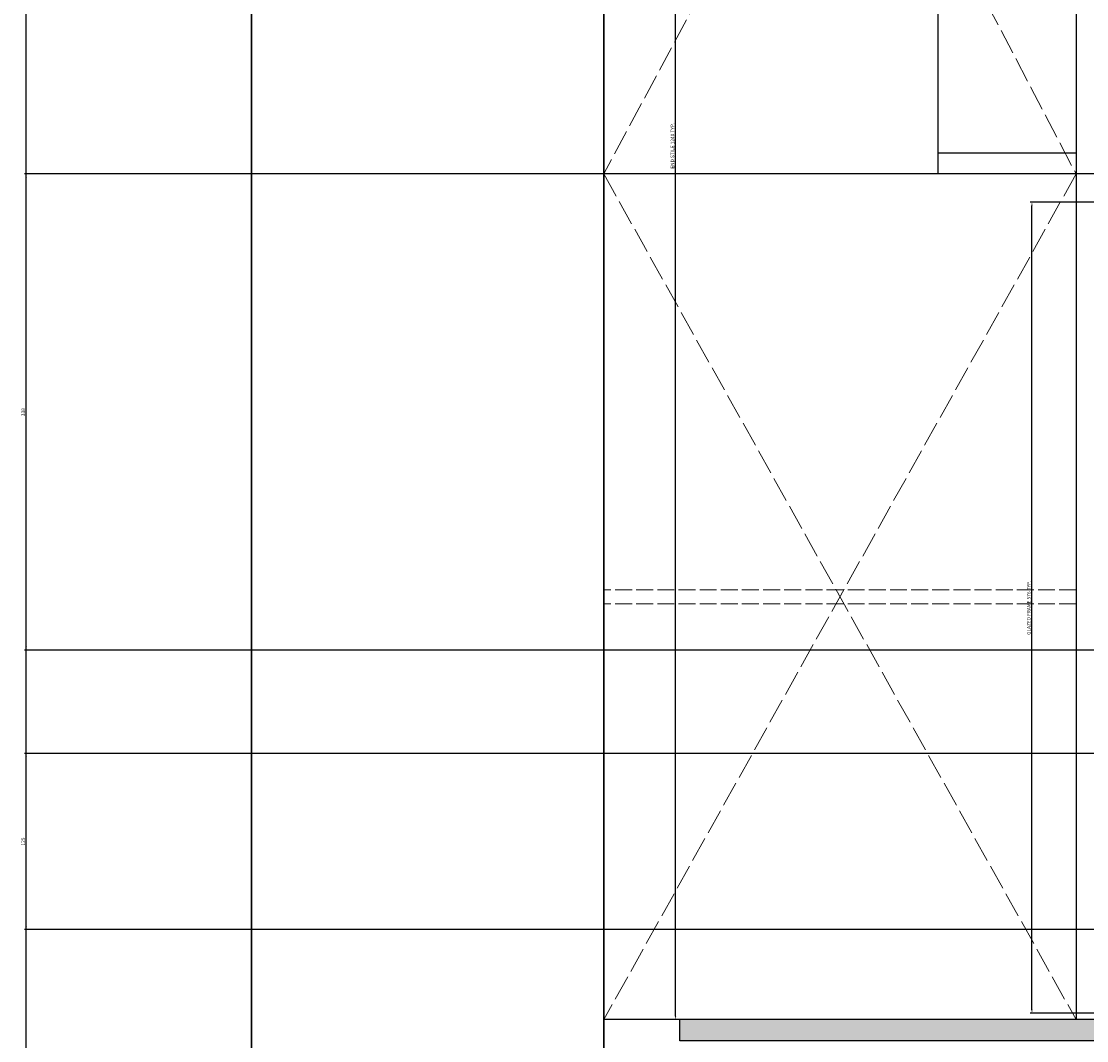
# Model space of a CAD drawing. Units: millimetres. Extents: x 2332 to 5836, y -853 to 2199.
# Tile 2 of 16: x 2332 to 3088, y 753 to 1476. Entities that reach past the tile are written whole.
import ezdxf

# ---------------------------------------------------------------- set-up
doc = ezdxf.new("R2010")
doc.units = ezdxf.units.MM
doc.linetypes.add('ACAD_ISO02W100', pattern=[15, 12, -3])
doc.layers.get('0').update_dxf_attribs({"color": 8})
for name, color, linetype, lineweight in [('A-ANNO-DIMS', 2, 'Continuous', 18), ('A-CSWK-HIDN', 8, 'ACAD_ISO02W100', 13), ('A-CSWK-PATT', 40, 'Continuous', 13), ('A-WALL', 8, 'Continuous', 30), ('SHELF', 40, 'Continuous', 25)]:
    doc.layers.add(name, color=color, linetype=linetype, lineweight=lineweight)
doc.styles.get("Standard").update_dxf_attribs({"font": 'arial.ttf'})
doc.dimstyles.new('ISO-25', dxfattribs={"dimtxt": 2.5, "dimasz": 2.5, "dimexe": 1.25, "dimexo": 0.625, "dimtad": 1, "dimtxsty": 'Standard', "dimcen": 2.5, "dimadec": 0, "dimazin": 0, "dimtfac": 1, "dimtmove": 0, "dimatfit": 3, "dimfxl": 1, "dimarcsym": 0})

# ---------------------------------------------------------------- blocks, each defined once
blk = doc.blocks.new('CAB-END-STILE')
for p, q in [((0, 1240), (0, 600)), ((98.09, 1240), (98.09, 0)), ((0, 615), (98.09, 615))]:
    blk.add_line(p, q)
blk = doc.blocks.new('*D11')
at = {"layer": 'A-ANNO-DIMS', "color": 0, "lineweight": -2, "transparency": 16777216}
for p, q in [((2981.33, 2007.8), (2794.7, 2007.8)), ((2795.95, 770.3), (2795.95, 2005.3)), ((2981.33, 767.8), (2794.7, 767.8))]:
    blk.add_line(p, q, dxfattribs=at)
at = {"layer": 'A-ANNO-DIMS', "color": 0, "transparency": 16777216}
for points in [[(2795.53, 2005.3), (2796.37, 2005.3), (2795.95, 2007.8)], [(2795.53, 770.3), (2796.37, 770.3), (2795.95, 767.8)]]:
    blk.add_solid(points, dxfattribs=at)
at = {"layer": 'Defpoints', "color": 0, "transparency": 16777216}
for p in [(2795.95, 2007.8), (2981.95, 2007.8), (2981.95, 767.8)]:
    blk.add_point(p, dxfattribs=at)
at = {"layer": 'A-ANNO-DIMS', "color": 0, "transparency": 16777216, "insert": (2794.03, 1387.8), "char_height": 2.5, "attachment_point": 5, "rotation": 90}
blk.add_mtext('END STILE 1240 TYP.', dxfattribs=at)
blk = doc.blocks.new('*D13')
at = {"layer": 'A-ANNO-DIMS', "color": 0, "lineweight": -2, "transparency": 16777216}
for p, q in [((3134.41, 1347.8), (3047.46, 1347.8)), ((3048.71, 774.77), (3048.71, 1345.3)), ((3134.41, 772.27), (3047.46, 772.27))]:
    blk.add_line(p, q, dxfattribs=at)
at = {"layer": 'A-ANNO-DIMS', "color": 0, "transparency": 16777216}
for points in [[(3048.29, 1345.3), (3049.13, 1345.3), (3048.71, 1347.8)], [(3048.29, 774.77), (3049.13, 774.77), (3048.71, 772.27)]]:
    blk.add_solid(points, dxfattribs=at)
at = {"layer": 'Defpoints', "color": 0, "transparency": 16777216}
for p in [(3048.71, 1347.8), (3135.04, 1347.8), (3135.04, 772.27)]:
    blk.add_point(p, dxfattribs=at)
at = {"layer": 'A-ANNO-DIMS', "color": 0, "transparency": 16777216, "insert": (3046.79, 1060.04), "char_height": 2.5, "attachment_point": 5, "rotation": 90}
blk.add_mtext('GLAZED FRAME 576 TYP.', dxfattribs=at)
blk = doc.blocks.new('*D16')
at = {"layer": 'A-ANNO-DIMS', "color": 0, "lineweight": -2, "transparency": 16777216}
for p, q in [((2494.41, 2007.8), (2334.14, 2007.8)), ((2335.39, -689.7), (2335.39, 2005.3)), ((2494.41, -692.2), (2334.14, -692.2))]:
    blk.add_line(p, q, dxfattribs=at)
at = {"layer": 'A-ANNO-DIMS', "color": 0, "transparency": 16777216}
for points in [[(2334.97, 2005.3), (2335.81, 2005.3), (2335.39, 2007.8)], [(2334.97, -689.7), (2335.81, -689.7), (2335.39, -692.2)]]:
    blk.add_solid(points, dxfattribs=at)
at = {"layer": 'Defpoints', "color": 0, "transparency": 16777216}
for p in [(2335.39, 2007.8), (2495.04, 2007.8), (2495.04, -692.2)]:
    blk.add_point(p, dxfattribs=at)
at = {"layer": 'A-ANNO-DIMS', "color": 0, "transparency": 16777216, "insert": (2333.49, 657.8), "char_height": 2.5, "attachment_point": 5, "rotation": 90}
blk.add_mtext('2700', dxfattribs=at)
blk = doc.blocks.new('*D28')
at = {"layer": 'A-ANNO-DIMS', "color": 0, "lineweight": -2, "transparency": 16777216}
for p, q in [((3772.04, 956.62), (2334.14, 956.62)), ((2335.39, 834.12), (2335.39, 954.12)), ((3772.04, 831.62), (2334.14, 831.62))]:
    blk.add_line(p, q, dxfattribs=at)
at = {"layer": 'A-ANNO-DIMS', "color": 0, "transparency": 16777216}
for points in [[(2334.97, 954.12), (2335.81, 954.12), (2335.39, 956.62)], [(2334.97, 834.12), (2335.81, 834.12), (2335.39, 831.62)]]:
    blk.add_solid(points, dxfattribs=at)
at = {"layer": 'Defpoints', "color": 0, "transparency": 16777216}
for p in [(2335.39, 956.62), (3772.66, 956.62), (3772.66, 831.62)]:
    blk.add_point(p, dxfattribs=at)
at = {"layer": 'A-ANNO-DIMS', "color": 0, "transparency": 16777216, "insert": (2333.49, 894.12), "char_height": 2.5, "attachment_point": 5, "rotation": 90}
blk.add_mtext('125', dxfattribs=at)
blk = doc.blocks.new('*D29')
at = {"layer": 'A-ANNO-DIMS', "color": 0, "lineweight": -2, "transparency": 16777216}
for p, q in [((3634.41, 1367.8), (2334.14, 1367.8)), ((2335.39, 1032.3), (2335.39, 1365.3)), ((3645.84, 1029.8), (2334.14, 1029.8))]:
    blk.add_line(p, q, dxfattribs=at)
at = {"layer": 'A-ANNO-DIMS', "color": 0, "transparency": 16777216}
for points in [[(2334.97, 1365.3), (2335.81, 1365.3), (2335.39, 1367.8)], [(2334.97, 1032.3), (2335.81, 1032.3), (2335.39, 1029.8)]]:
    blk.add_solid(points, dxfattribs=at)
at = {"layer": 'Defpoints', "color": 0, "transparency": 16777216}
for p in [(2335.39, 1367.8), (3635.04, 1367.8), (3646.47, 1029.8)]:
    blk.add_point(p, dxfattribs=at)
at = {"layer": 'A-ANNO-DIMS', "color": 0, "transparency": 16777216, "insert": (2333.49, 1198.8), "char_height": 2.5, "attachment_point": 5, "rotation": 90}
blk.add_mtext('338', dxfattribs=at)

msp = doc.modelspace()

# ---------------------------------------------------------------- hatches: boundary and pattern name
at = {"layer": 'A-CSWK-PATT'}
h = msp.add_hatch(color=256, dxfattribs=at)
h.dxf.hatch_style = 1
h.paths.add_polyline_path([(3635.04, 767.803), (3135.04, 767.803), (3095.04, 767.803), (2798.91, 767.803), (2798.91, 752.803), (3635.04, 752.803)])

# ---------------------------------------------------------------- linework, layer by layer
at = {"layer": 'A-CSWK-HIDN', "ltscale": 1.5}
for p, q in [((2745.04, 2007.803), (3080.04, 1367.803)), ((3080.04, 1992.803), (2745.04, 1367.803)), ((2745.04, 1367.803), (3080.04, 767.803)), ((3080.04, 1367.803), (2745.04, 767.803))]:
    msp.add_line(p, q, dxfattribs=at)
at = {"layer": 'A-CSWK-HIDN'}
for p, q in [((3080.04, 1072.803), (2745.04, 1072.803)), ((3080.04, 1062.803), (2745.04, 1062.803))]:
    msp.add_line(p, q, dxfattribs=at)
at = {"layer": 'A-WALL'}
for p, q in [((2495.04, -692.197), (2495.04, 2007.803)), ((2745.04, -692.197), (2745.04, 2007.803))]:
    msp.add_line(p, q, dxfattribs=at)
at = {"layer": 'SHELF'}
for p, q in [((3635.04, 1367.803), (2745.04, 1367.803)), ((3095.04, 767.803), (2745.04, 767.803)), ((2798.91, 752.803), (2798.91, 767.803)), ((3635.04, 752.803), (2798.91, 752.803))]:
    msp.add_line(p, q, dxfattribs=at)

# ---------------------------------------------------------------- block references
msp.add_blockref('CAB-END-STILE', (2981.95, 767.803), dxfattribs=at)

# ---------------------------------------------------------------- dimensions: what is measured, and where the dimension line sits
at = {"layer": 'A-ANNO-DIMS'}
for base, p1, p2, picture, middle in [((2335.39, 2007.803), (2495.04, -692.197), (2495.04, 2007.803), '*D16', (2333.488, 657.803)), ((2335.39, 1367.803), (3646.468, 1029.801), (3635.04, 1367.803), '*D29', (2333.488, 1198.802)), ((2335.39, 956.62), (3772.661, 831.62), (3772.661, 956.62), '*D28', (2333.488, 894.12))]:
    dim = msp.add_linear_dim(base=base, p1=p1, p2=p2, angle=90, dimstyle='ISO-25', override={"dimdec": 0, "dimlfac": 1, "dimrnd": 0, "dimzin": 0, "dimdsep": 46, "dimlunit": 2}, dxfattribs=at)
    dim.commit()
    dim.dimension.update_dxf_attribs({"geometry": picture, "text_midpoint": middle})
for base, p1, p2, text, picture, middle in [((2795.95, 2007.803), (2981.95, 767.803), (2981.95, 2007.803), 'END STILE <> TYP.', '*D11', (2794.032, 1387.803)), ((3048.71, 1347.803), (3135.04, 772.269), (3135.04, 1347.803), 'GLAZED FRAME <> TYP.', '*D13', (3046.792, 1060.036))]:
    dim = msp.add_linear_dim(base=base, p1=p1, p2=p2, angle=90, text=text, dimstyle='ISO-25', override={"dimdec": 0, "dimlfac": 1, "dimrnd": 0, "dimzin": 0, "dimdsep": 46, "dimlunit": 2}, dxfattribs=at)
    dim.commit()
    dim.dimension.update_dxf_attribs({"geometry": picture, "text_midpoint": middle})

doc.saveas('drawing.dxf')
